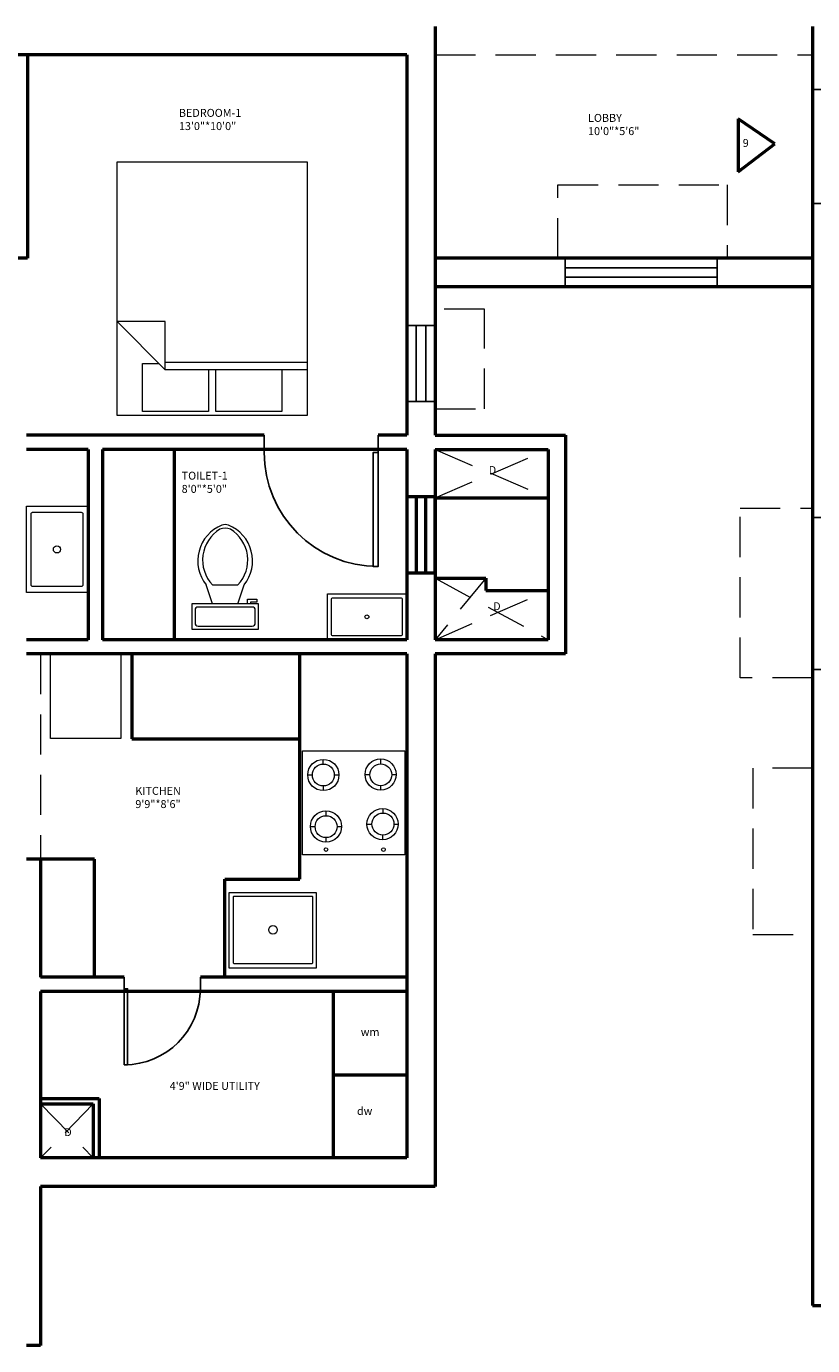
# Model space of a CAD drawing. Units: inches. Extents: x 291 to 2631, y 456 to 2623.
# Tile 8 of 22: x 1861 to 2109, y 515 to 931. Entities that reach past the tile are written whole.
import ezdxf

# ---------------------------------------------------------------- set-up
doc = ezdxf.new("R2010")
doc.units = ezdxf.units.IN
doc.linetypes.add('DASHED', pattern=[19.05, 12.7, -6.35])
for name, color, linetype, lineweight in [('A-ANNO-TEXT', 3, 'Continuous', 25), ('A-AREA-IDEN', 7, 'Continuous', 25), ('A-DOOR', 3, 'Continuous', 25), ('A-EQPM', 8, 'Continuous', 18), ('A-FLOR-FIXT', 9, 'Continuous', 18), ('A-FLOR-OVHD', 1, 'DASHED', 18), ('A-FURN', 8, 'Continuous', 18), ('A-GLAZ', 4, 'Continuous', 25), ('A-WALL', 7, 'Continuous', 50)]:
    doc.layers.add(name, color=color, linetype=linetype, lineweight=lineweight)
doc.styles.get("Standard").update_dxf_attribs({"font": 'arial.ttf'})

# ---------------------------------------------------------------- blocks, each defined once
blk = doc.blocks.new('*U2')
for p, q in [((0, 0), (0, -6)), ((40, 0), (40, -6))]:
    blk.add_line(p, q)
blk.add_lwpolyline([(0, 0), (0, 40), (1.75, 40), (1.75, 0)], close=True)
blk.add_arc((0, 0), 40, 0, 90)
blk = doc.blocks.new('Bed - Queen')
for p, q in [((0, -80.00003), (0, 0)), ((0, 0), (59.99999, 0)), ((59.99999, 0), (59.99999, -80.00003)), ((7.99999, -1.2), (28.79998, -1.2)), ((7.99999, -14.4), (7.99999, -1.2)), ((28.79998, -1.2), (28.79998, -14.4)), ((31.19999, -1.2), (51.99999, -1.2)), ((31.19999, -14.4), (31.19999, -1.2)), ((51.99999, -1.2), (51.99999, -16.4)), ((0, -14.4), (44.8, -14.4)), ((59.99999, -29.6), (44.8, -14.4)), ((44.8, -14.4), (44.8, -29.6)), ((51.99999, -16.4), (46.79936, -16.4)), ((44.8, -16.8), (0, -16.8)), ((44.8, -29.6), (59.99999, -29.6)), ((59.99999, -80.00003), (0, -80.00003))]:
    blk.add_line(p, q)
blk = doc.blocks.new('Toilet - top')
for p, q in [((9.5, -6), (9.5, -2)), ((-8, -8.5), (-8, -8)), ((-7, -8), (-7, -9.5)), ((-4, -8), (-6, -14)), ((4, -8), (6, -14)), ((-10, -8.5), (-8, -8.5)), ((-10, -9.5), (-10, -8.5)), ((-7, -9.5), (-10, -9.5)), ((4, -14), (-4, -14))]:
    blk.add_line(p, q)
blk.add_lwpolyline([(10.5, -8), (10.5, 0), (-10.5, 0), (-10.5, -8)], close=True)
for points in [[(-9.5, -2), (-9.5, -6)], [(8.5, -1), (-8.5, -1)], [(-8.5, -7), (8.5, -7)]]:
    blk.add_lwpolyline(points)
for centre, radius, start, end in [((-8.62, -1.88), 0.884, 81.8699, 188.1301), ((8.62, -1.88), 0.884, 351.8699, 98.1301), ((-8.62, -6.12), 0.884, 171.8699, 278.1301), ((8.62, -6.12), 0.884, 261.8699, 8.1301), ((3.52, -21.58), 12.17, 141.4691, 247.9714), ((4.2, -21.82), 11.33, 136.3677, 238.9468), ((-3.52, -21.58), 12.17, 292.0284, 38.5307), ((-4.2, -21.82), 11.33, 301.053, 43.6321), ((0, -27.88), 4, 245.7318, 294.2682), ((0, -29), 4, 254.8605, 285.1395)]:
    blk.add_arc(centre, radius, start, end)
blk = doc.blocks.new('WIN-1200')
for p, q in [((0, 0), (0, 48)), ((0, 48), (9, 48)), ((3, 0), (3, 48)), ((6, 48), (6, 0)), ((9, 48), (9, 0)), ((9, 0), (0, 0))]:
    blk.add_line(p, q)
blk = doc.blocks.new('COOKTOP')
for p, q in [((6.54, 28.68), (6.54, 30.14)), ((24.62, 30.31), (24.62, 28.76)), ((1.62, 25.22), (3.08, 25.22)), ((10, 25.22), (11.46, 25.22)), ((19.7, 25.39), (21.21, 25.39)), ((28.13, 25.39), (29.54, 25.39)), ((6.54, 21.76), (6.54, 20.3)), ((24.62, 21.83), (24.62, 20.47)), ((7.38, 13.92), (7.38, 12.38)), ((25.35, 14.65), (25.34, 13.21)), ((2.46, 9), (3.95, 9)), ((10.87, 9), (12.3, 9)), ((20.32, 9.73), (21.89, 9.73)), ((28.81, 9.73), (30.16, 9.73)), ((7.38, 5.46), (7.38, 4.08)), ((25.26, 6.28), (25.24, 4.81))]:
    blk.add_line(p, q)
blk.add_lwpolyline([(0, 32.79), (32.25, 32.79), (32.25, 0), (0, 0)], close=True)
for centre, radius in [((6.54, 25.22), 4.92), ((24.62, 25.39), 4.92), ((6.54, 25.22), 3.46), ((24.67, 25.29), 3.46), ((7.38, 9), 4.92), ((25.24, 9.73), 4.92), ((25.35, 9.74), 3.46), ((7.41, 8.92), 3.46), ((7.38, 1.69), 0.572), ((25.5, 1.69), 0.572)]:
    blk.add_circle(centre, radius)
blk = doc.blocks.new('WIN-600')
for p, q in [((24, 9), (0, 9)), ((0, 9), (0, 0)), ((24, 0), (24, 9)), ((24, 6), (0, 6)), ((0, 3), (24, 3)), ((0, 0), (24, 0))]:
    blk.add_line(p, q)

msp = doc.modelspace()

# ---------------------------------------------------------------- linework, layer by layer
at = {"layer": 'A-FLOR-OVHD'}
for p, q in [((1989.87, 921.98), (2108.97, 921.98)), ((2028.62, 857.82), (2028.62, 880.98)), ((2028.62, 880.98), (2082.05, 880.98)), ((2082.05, 880.98), (2082.05, 857.82)), ((2005.4, 841.81), (1989.87, 841.81)), ((2005.4, 810.34), (2005.4, 841.81)), ((1989.87, 810.34), (2005.4, 810.34)), ((1989.87, 797.48), (2025.47, 782.24)), ((1989.87, 782.24), (2025.47, 797.48)), ((2086.08, 725.45), (2086.08, 778.93)), ((2086.08, 778.93), (2108.97, 778.93)), ((1989.87, 756.92), (2025.47, 737.48)), ((2005.84, 756.92), (1989.87, 737.48)), ((1989.87, 737.48), (2025.47, 753.05)), ((1865.37, 732.98), (1865.37, 668.21)), ((2108.97, 725.45), (2086.08, 725.45)), ((2108.97, 696.94), (2090.11, 696.94)), ((2090.11, 696.94), (2090.11, 644.53)), ((2090.11, 644.53), (2108.97, 644.53)), ((1865.37, 591.05), (1881.94, 573.98)), ((1881.94, 591.05), (1865.37, 573.98))]:
    msp.add_line(p, q, dxfattribs=at)
at = {"layer": 'A-FURN'}
for points in [[(1860.87, 779.65), (1880.37, 779.65), (1880.37, 752.33), (1860.87, 752.33)], [(1980.87, 737.48), (1955.88, 737.48), (1955.88, 752), (1980.87, 752)], [(1868.45, 732.98), (1890.7, 732.98), (1890.7, 706.27), (1868.45, 706.27)], [(1924.9, 657.72), (1952.34, 657.72), (1952.34, 633.82), (1924.9, 633.82)]]:
    msp.add_lwpolyline(points, close=True, dxfattribs=at)
for points in [[(1862.85, 777.67), (1878.2, 777.67, -0.414214), (1878.7, 777.17), (1878.7, 754.78, -0.414214), (1878.2, 754.28), (1862.85, 754.28, -0.414214), (1862.35, 754.78), (1862.35, 777.17, -0.414214)], [(1957.66, 750.69), (1978.97, 750.69, -0.414214), (1979.47, 750.19), (1979.47, 739.2, -0.414214), (1978.97, 738.7), (1957.66, 738.7, -0.414214), (1957.16, 739.2), (1957.16, 750.19, -0.414214)], [(1926.54, 656.61), (1950.84, 656.61, -0.414214), (1951.14, 656.31), (1951.14, 635.53, -0.414214), (1950.84, 635.23), (1926.54, 635.23, -0.414214), (1926.24, 635.53), (1926.24, 656.31, -0.414214)]]:
    msp.add_lwpolyline(points, format="xyb", close=True, dxfattribs=at)
for centre, radius in [((1870.52, 765.98), 1.14), ((1968.32, 744.69), 0.607), ((1938.69, 645.92), 1.36)]:
    msp.add_circle(centre, radius, dxfattribs=at)
at = {"layer": 'A-WALL'}
for p, q in [((1989.87, 930.98), (1989.87, 801.98)), ((2108.97, 930.98), (2108.97, 527.48)), ((1980.87, 921.98), (1604.37, 921.98)), ((1861.27, 921.98), (1861.27, 857.84)), ((1980.87, 921.98), (1980.87, 801.98)), ((2085.43, 901.8), (2085.43, 885.12)), ((2097.05, 893.96), (2085.43, 901.8)), ((2085.43, 885.12), (2097.05, 893.96)), ((1861.27, 857.84), (1824.87, 857.84)), ((2108.97, 857.82), (1989.87, 857.82)), ((2108.97, 848.82), (1989.87, 848.82)), ((1935.89, 801.98), (1860.87, 801.98)), ((1980.87, 801.98), (1971.89, 801.98)), ((1989.87, 801.98), (2031.03, 801.98)), ((2031.03, 801.98), (2031.03, 732.98)), ((1880.37, 797.48), (1860.87, 797.48)), ((1880.37, 797.48), (1880.37, 737.48)), ((1980.87, 797.48), (1884.87, 797.48)), ((1884.87, 797.48), (1884.87, 737.48)), ((1907.52, 797.48), (1907.52, 737.48)), ((1980.87, 797.48), (1980.87, 737.48)), ((1989.87, 797.48), (2025.47, 797.48)), ((1989.87, 797.48), (1989.87, 737.48)), ((2025.47, 797.48), (2025.47, 737.48)), ((1989.87, 782.53), (1980.87, 782.53)), ((1980.87, 782.53), (1980.87, 758.53)), ((1983.87, 782.53), (1983.87, 758.53)), ((1986.87, 758.53), (1986.87, 782.53)), ((1989.87, 758.53), (1989.87, 782.53)), ((1989.87, 782.24), (2025.47, 782.24)), ((1980.87, 758.53), (1989.87, 758.53)), ((1989.87, 756.92), (2005.84, 756.92)), ((2005.84, 756.92), (2005.84, 753.05)), ((2005.84, 753.05), (2025.47, 753.05)), ((1880.37, 737.48), (1860.87, 737.48)), ((1980.87, 737.48), (1884.87, 737.48)), ((2025.47, 737.48), (1989.87, 737.48)), ((1980.87, 732.98), (1860.87, 732.98)), ((1894.17, 732.98), (1894.17, 706.2)), ((1947.15, 661.96), (1947.15, 732.98)), ((1980.87, 732.98), (1980.87, 573.98)), ((2031.03, 732.98), (1989.87, 732.98)), ((1989.87, 732.98), (1989.87, 564.98)), ((1894.17, 706.2), (1947.15, 706.2)), ((1882.34, 668.21), (1860.87, 668.21)), ((1865.37, 668.21), (1865.37, 630.98)), ((1882.34, 630.98), (1882.34, 668.21)), ((1923.51, 630.98), (1923.51, 661.96)), ((1923.51, 661.96), (1947.15, 661.96)), ((1891.77, 630.98), (1865.37, 630.98)), ((1980.87, 630.98), (1915.77, 630.98)), ((1980.87, 626.48), (1865.37, 626.48)), ((1865.37, 626.48), (1865.37, 573.98)), ((1957.71, 626.48), (1957.71, 573.98)), ((1957.71, 600.23), (1980.87, 600.23)), ((1865.37, 592.73), (1883.79, 592.73)), ((1865.37, 591.05), (1881.94, 591.05)), ((1881.94, 591.05), (1881.94, 573.98)), ((1883.79, 592.73), (1883.79, 573.98)), ((1980.87, 573.98), (1865.37, 573.98)), ((1989.87, 564.98), (1865.37, 564.98)), ((1865.37, 564.98), (1865.37, 514.78)), ((2108.97, 527.48), (2251.97, 527.48)), ((1865.37, 514.78), (1860.87, 514.78))]:
    msp.add_line(p, q, dxfattribs=at)

# ---------------------------------------------------------------- block references
at = {"layer": 'A-DOOR'}
for p, xscale, yscale, zscale, rotation in [((2114.37, 911.1), 0.9, 0.9, 0.9, 270), ((1971.89, 796.58), 0.9, 0.9, 0.9, 180), ((1891.77, 627.38), -0.6, 0.6, 0.6, 180)]:
    msp.add_blockref('*U2', p, dxfattribs=dict(at, xscale=xscale, yscale=yscale, zscale=zscale, rotation=rotation))
at = {"layer": 'A-EQPM'}
msp.add_blockref('COOKTOP', (1948.03, 669.58), dxfattribs=at)
at = {"layer": 'A-FLOR-FIXT', "rotation": 180}
msp.add_blockref('Toilet - top', (1923.6, 740.78), dxfattribs=at)
at = {"layer": 'A-FURN', "rotation": 180}
msp.add_blockref('Bed - Queen', (1949.49, 808.26), dxfattribs=at)
at = {"layer": 'A-GLAZ'}
for name, p, rotation in [('WIN-1200', (2078.9, 848.82), 90.00000000000007), ('WIN-600', (1980.87, 836.63), 269.999999999999), ('WIN-1200', (2117.97, 776.04), 180)]:
    msp.add_blockref(name, p, dxfattribs=dict(at, rotation=rotation))

# ---------------------------------------------------------------- texts
at = {"layer": 'A-ANNO-TEXT', "char_height": 2.5, "attachment_point": 1}
for s, width, insert in [('9', 4.318, (2086.92, 895.45)), ('D', 2.3445, (2006.77, 792.28)), ('D', 2.5794, (2008.17, 749.29)), ('wm', 14.6196, (1966.39, 614.97)), ('dw', 9.8141, (1965.19, 590.06)), ('D', 2.2917, (1872.82, 583.37))]:
    msp.add_mtext_dynamic_manual_height_columns(s, width=width, gutter_width=12.5, heights=[0], dxfattribs=dict(at, insert=insert))
at = {"layer": 'A-AREA-IDEN', "char_height": 2.5, "attachment_point": 1}
for s, width, insert in [('BEDROOM-1\\P13\'0"*10\'0"', 69.891, (1909.01, 904.94)), ('LOBBY\\P10\'0"*5\'6"', 64.6503, (2038.11, 903.35)), ('TOILET-1\\P8\'0"*5\'0"', 23.782, (1909.87, 790.48)), ('KITCHEN\\P9\'9"*8\'6"', 46.3722, (1895.25, 691.04)), ('4\'9" WIDE UTILITY', 61.7967, (1906.1, 597.96))]:
    msp.add_mtext_dynamic_manual_height_columns(s, width=width, gutter_width=12.5, heights=[0], dxfattribs=dict(at, insert=insert))

doc.saveas('drawing.dxf')
